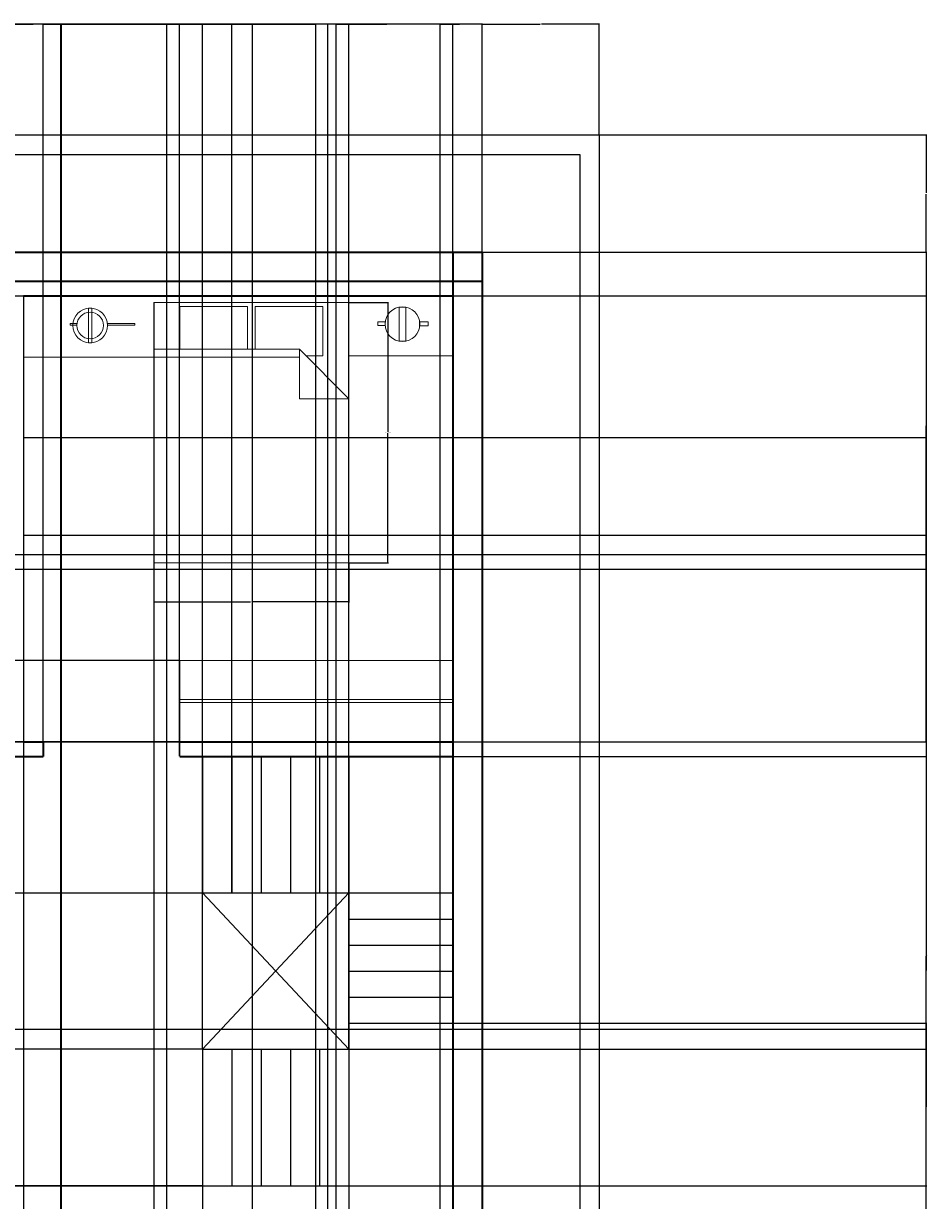
# Model space of a CAD drawing. Units: inches. Extents: x -47 to 496, y -43 to 706.
# Tile 6 of 6: x 218 to 496, y 344 to 706. Entities that reach past the tile are written whole.
import ezdxf

# ---------------------------------------------------------------- set-up
doc = ezdxf.new("R2010")
doc.units = ezdxf.units.IN
doc.linetypes.add('ACAD_ISO02W100', pattern=[15, 12, -3])
for name, color, linetype, lineweight in [('A-ANNO-DIMS', 2, 'Continuous', 18), ('A-FLOR-CASE', 3, 'Continuous', 18), ('A-FLOR-STRS-HIDN', 6, 'ACAD_ISO02W100', 18), ('C-PROP', 7, 'Continuous', 25), ('FURNITURE', 3, 'Continuous', 18), ('STAIR CASE', 6, 'Continuous', 25), ('WALL', 7, 'Continuous', 35)]:
    doc.layers.add(name, color=color, linetype=linetype, lineweight=lineweight)
doc.styles.get("Standard").update_dxf_attribs({"font": 'arial.ttf'})
doc.dimstyles.get("Standard").update_dxf_attribs({"dimtxt": 0.18, "dimasz": 0.18, "dimexe": 0.18, "dimexo": 0.0625, "dimgap": 0.09, "dimtad": 0, "dimtih": 1, "dimtoh": 1, "dimdec": 4, "dimzin": 0, "dimdsep": 46, "dimtxsty": 'Standard', "dimcen": 0.09, "dimadec": 0, "dimazin": 0, "dimtfac": 1, "dimtdec": 4, "dimtofl": 0, "dimtmove": 0, "dimatfit": 3, "dimfxl": 1, "dimtolj": 1, "dimtzin": 0, "dimarcsym": 0})

# ---------------------------------------------------------------- blocks, each defined once
blk = doc.blocks.new('Bed - Queen')
for p, q in [((0, -80.00003), (0, 0)), ((0, 0), (59.99999, 0)), ((59.99999, 0), (59.99999, -80.00003)), ((7.99999, -1.2), (28.79998, -1.2)), ((7.99999, -14.4), (7.99999, -1.2)), ((28.79998, -1.2), (28.79998, -14.4)), ((31.19999, -1.2), (51.99999, -1.2)), ((31.19999, -14.4), (31.19999, -1.2)), ((51.99999, -1.2), (51.99999, -16.4)), ((0, -14.4), (44.8, -14.4)), ((59.99999, -29.6), (44.8, -14.4)), ((44.8, -14.4), (44.8, -29.6)), ((44.8, -16.8), (0, -16.8)), ((51.99999, -16.4), (46.79936, -16.4)), ((44.8, -29.6), (59.99999, -29.6)), ((59.99999, -80.00003), (0, -80.00003))]:
    blk.add_line(p, q)
blk = doc.blocks.new('*D10')
at = {"layer": 'A-ANNO-DIMS', "color": 0, "lineweight": -2, "transparency": 16777216}
for p, q in [((318.53, 619.97), (330.64, 619.97)), ((330.46, 619.79), (330.46, 580.16)), ((330.46, 540.15), (330.46, 579.78)), ((318.53, 539.97), (330.64, 539.97))]:
    blk.add_line(p, q, dxfattribs=at)
at = {"layer": 'A-ANNO-DIMS', "color": 0, "transparency": 16777216}
for points in [[(330.43, 619.79), (330.49, 619.79), (330.46, 619.97)], [(330.43, 540.15), (330.49, 540.15), (330.46, 539.97)]]:
    blk.add_solid(points, dxfattribs=at)
at = {"layer": 'Defpoints', "color": 0, "transparency": 16777216}
for p in [(318.46, 619.97), (330.46, 619.97), (318.46, 539.97)]:
    blk.add_point(p, dxfattribs=at)
at = {"layer": 'A-ANNO-DIMS', "color": 0, "transparency": 16777216, "insert": (330.46, 579.97), "char_height": 0.18, "attachment_point": 5}
blk.add_mtext('\\A1;QUEEN BED 80', dxfattribs=at)
blk = doc.blocks.new('*D11')
at = {"layer": 'A-ANNO-DIMS', "color": 0, "lineweight": -2, "transparency": 16777216}
for p, q in [((258.46, 539.91), (258.46, 527.79)), ((318.46, 539.91), (318.46, 527.79)), ((258.64, 527.97), (288.24, 527.97)), ((318.28, 527.97), (288.68, 527.97))]:
    blk.add_line(p, q, dxfattribs=at)
at = {"layer": 'A-ANNO-DIMS', "color": 0, "transparency": 16777216}
for points in [[(258.64, 528), (258.64, 527.94), (258.46, 527.97)], [(318.28, 528), (318.28, 527.94), (318.46, 527.97)]]:
    blk.add_solid(points, dxfattribs=at)
at = {"layer": 'Defpoints', "color": 0, "transparency": 16777216}
for p in [(258.46, 539.97), (318.46, 539.97), (318.46, 527.97)]:
    blk.add_point(p, dxfattribs=at)
at = {"layer": 'A-ANNO-DIMS', "color": 0, "transparency": 16777216, "insert": (288.46, 527.97), "char_height": 0.18, "attachment_point": 5}
blk.add_mtext('\\A1;60', dxfattribs=at)
blk = doc.blocks.new('*D16')
at = {"layer": 'A-ANNO-DIMS', "color": 0, "lineweight": -2, "transparency": 16777216}
for p, q in [((359.45, 635.53), (359.45, 705.7)), ((359.63, 705.52), (377.24, 705.52)), ((395.27, 705.52), (377.67, 705.52)), ((395.45, 671.53), (395.45, 705.7))]:
    blk.add_line(p, q, dxfattribs=at)
at = {"layer": 'A-ANNO-DIMS', "color": 0, "transparency": 16777216}
for points in [[(359.63, 705.55), (359.63, 705.49), (359.45, 705.52)], [(395.27, 705.55), (395.27, 705.49), (395.45, 705.52)]]:
    blk.add_solid(points, dxfattribs=at)
at = {"layer": 'Defpoints', "color": 0, "transparency": 16777216}
for p in [(395.45, 705.52), (395.45, 671.47), (359.45, 635.47)]:
    blk.add_point(p, dxfattribs=at)
at = {"layer": 'A-ANNO-DIMS', "color": 0, "transparency": 16777216, "insert": (377.45, 705.52), "char_height": 0.18, "attachment_point": 5}
blk.add_mtext('\\A1;36', dxfattribs=at)
blk = doc.blocks.new('*D17')
at = {"layer": 'A-ANNO-DIMS', "color": 0, "lineweight": -2, "transparency": 16777216}
for p, q in [((395.52, 671.47), (496.14, 671.47)), ((495.96, 671.29), (495.96, 653.65)), ((495.96, 635.65), (495.96, 653.29)), ((359.52, 635.47), (496.14, 635.47))]:
    blk.add_line(p, q, dxfattribs=at)
at = {"layer": 'A-ANNO-DIMS', "color": 0, "transparency": 16777216}
for points in [[(495.93, 671.29), (495.99, 671.29), (495.96, 671.47)], [(495.93, 635.65), (495.99, 635.65), (495.96, 635.47)]]:
    blk.add_solid(points, dxfattribs=at)
at = {"layer": 'Defpoints', "color": 0, "transparency": 16777216}
for p in [(395.45, 671.47), (495.96, 671.47), (359.45, 635.47)]:
    blk.add_point(p, dxfattribs=at)
at = {"layer": 'A-ANNO-DIMS', "color": 0, "transparency": 16777216, "insert": (495.96, 653.47), "char_height": 0.18, "attachment_point": 5}
blk.add_mtext('\\A1;36', dxfattribs=at)
blk = doc.blocks.new('*D18')
at = {"layer": 'A-ANNO-DIMS', "color": 0, "lineweight": -2, "transparency": 16777216}
for p, q in [((359.52, 635.47), (496.14, 635.47)), ((495.96, 635.29), (495.96, 419.4)), ((495.96, 203.15), (495.96, 419.04)), ((359.52, 202.97), (496.14, 202.97))]:
    blk.add_line(p, q, dxfattribs=at)
at = {"layer": 'A-ANNO-DIMS', "color": 0, "transparency": 16777216}
for points in [[(495.93, 635.29), (495.99, 635.29), (495.96, 635.47)], [(495.93, 203.15), (495.99, 203.15), (495.96, 202.97)]]:
    blk.add_solid(points, dxfattribs=at)
at = {"layer": 'Defpoints', "color": 0, "transparency": 16777216}
for p in [(359.45, 635.47), (495.96, 635.47), (359.45, 202.97)]:
    blk.add_point(p, dxfattribs=at)
at = {"layer": 'A-ANNO-DIMS', "color": 0, "transparency": 16777216, "insert": (495.96, 419.22), "char_height": 0.18, "attachment_point": 5}
blk.add_mtext('\\A1;432.5', dxfattribs=at)
blk = doc.blocks.new('*D22')
at = {"layer": 'A-ANNO-DIMS', "color": 0, "lineweight": -2, "transparency": 16777216}
for p, q in [((229.88, 163.9), (229.88, 705.7)), ((230.06, 705.52), (245.73, 705.52)), ((262.33, 705.52), (246.66, 705.52)), ((262.51, 163.9), (262.51, 705.7))]:
    blk.add_line(p, q, dxfattribs=at)
at = {"layer": 'A-ANNO-DIMS', "color": 0, "transparency": 16777216}
for points in [[(230.06, 705.55), (230.06, 705.49), (229.88, 705.52)], [(262.33, 705.55), (262.33, 705.49), (262.51, 705.52)]]:
    blk.add_solid(points, dxfattribs=at)
at = {"layer": 'Defpoints', "color": 0, "transparency": 16777216}
for p in [(262.51, 705.52), (229.88, 163.83), (262.51, 163.83)]:
    blk.add_point(p, dxfattribs=at)
at = {"layer": 'A-ANNO-DIMS', "color": 0, "transparency": 16777216, "insert": (246.2, 705.52), "char_height": 0.18, "attachment_point": 5}
blk.add_mtext('\\A1;32.636', dxfattribs=at)
blk = doc.blocks.new('*D24')
at = {"layer": 'A-ANNO-DIMS', "color": 0, "lineweight": -2, "transparency": 16777216}
for p, q in [((314.53, 186.25), (314.53, 705.7)), ((314.71, 705.52), (330.12, 705.52)), ((346.32, 705.52), (330.91, 705.52)), ((346.5, 186.25), (346.5, 705.7))]:
    blk.add_line(p, q, dxfattribs=at)
at = {"layer": 'A-ANNO-DIMS', "color": 0, "transparency": 16777216}
for points in [[(314.71, 705.55), (314.71, 705.49), (314.53, 705.52)], [(346.32, 705.55), (346.32, 705.49), (346.5, 705.52)]]:
    blk.add_solid(points, dxfattribs=at)
at = {"layer": 'Defpoints', "color": 0, "transparency": 16777216}
for p in [(346.5, 705.52), (314.53, 186.18), (346.5, 186.18)]:
    blk.add_point(p, dxfattribs=at)
at = {"layer": 'A-ANNO-DIMS', "color": 0, "transparency": 16777216, "insert": (330.52, 705.52), "char_height": 0.18, "attachment_point": 5}
blk.add_mtext('\\A1;31.97', dxfattribs=at)
blk = doc.blocks.new('*D26')
at = {"layer": 'A-ANNO-DIMS', "color": 0, "lineweight": -2, "transparency": 16777216}
for p, q in [((213.95, 131.03), (213.95, 705.7)), ((214.13, 705.52), (221.46, 705.52)), ((229.7, 705.52), (222.37, 705.52)), ((229.88, 163.9), (229.88, 705.7))]:
    blk.add_line(p, q, dxfattribs=at)
at = {"layer": 'A-ANNO-DIMS', "color": 0, "transparency": 16777216}
for points in [[(214.13, 705.55), (214.13, 705.49), (213.95, 705.52)], [(229.7, 705.55), (229.7, 705.49), (229.88, 705.52)]]:
    blk.add_solid(points, dxfattribs=at)
at = {"layer": 'Defpoints', "color": 0, "transparency": 16777216}
for p in [(229.88, 705.52), (229.88, 163.83), (213.95, 130.97)]:
    blk.add_point(p, dxfattribs=at)
at = {"layer": 'A-ANNO-DIMS', "color": 0, "transparency": 16777216, "insert": (221.92, 705.52), "char_height": 0.18, "attachment_point": 5}
blk.add_mtext('\\A1;15.924', dxfattribs=at)
blk = doc.blocks.new('*D28')
at = {"layer": 'A-ANNO-DIMS', "color": 0, "lineweight": -2, "transparency": 16777216}
for p, q in [((346.5, 165.93), (346.5, 705.7)), ((346.68, 705.52), (352.52, 705.52)), ((359.27, 705.52), (353.43, 705.52)), ((359.45, 131.03), (359.45, 705.7))]:
    blk.add_line(p, q, dxfattribs=at)
at = {"layer": 'A-ANNO-DIMS', "color": 0, "transparency": 16777216}
for points in [[(346.68, 705.55), (346.68, 705.49), (346.5, 705.52)], [(359.27, 705.55), (359.27, 705.49), (359.45, 705.52)]]:
    blk.add_solid(points, dxfattribs=at)
at = {"layer": 'Defpoints', "color": 0, "transparency": 16777216}
for p in [(359.45, 705.52), (346.5, 165.87), (359.45, 130.97)]:
    blk.add_point(p, dxfattribs=at)
at = {"layer": 'A-ANNO-DIMS', "color": 0, "transparency": 16777216, "insert": (352.98, 705.52), "char_height": 0.18, "attachment_point": 5}
blk.add_mtext('\\A1;12.954', dxfattribs=at)
blk = doc.blocks.new('*D32')
at = {"layer": 'A-ANNO-DIMS', "color": 0, "lineweight": -2, "transparency": 16777216}
for p, q in [((61.45, 635.53), (61.45, 705.7)), ((61.63, 705.52), (210.16, 705.52)), ((359.27, 705.52), (210.75, 705.52)), ((359.45, 635.53), (359.45, 705.7))]:
    blk.add_line(p, q, dxfattribs=at)
at = {"layer": 'A-ANNO-DIMS', "color": 0, "transparency": 16777216}
for points in [[(61.63, 705.55), (61.63, 705.49), (61.45, 705.52)], [(359.27, 705.55), (359.27, 705.49), (359.45, 705.52)]]:
    blk.add_solid(points, dxfattribs=at)
at = {"layer": 'Defpoints', "color": 0, "transparency": 16777216}
for p in [(359.45, 705.52), (61.45, 635.47), (359.45, 635.47)]:
    blk.add_point(p, dxfattribs=at)
at = {"layer": 'A-ANNO-DIMS', "color": 0, "transparency": 16777216, "insert": (210.45, 705.52), "char_height": 0.18, "attachment_point": 5}
blk.add_mtext('\\A1;298', dxfattribs=at)
blk = doc.blocks.new('*D35')
at = {"layer": 'A-ANNO-DIMS', "color": 0, "lineweight": -2, "transparency": 16777216}
for p, q in [((218.45, 484.91), (218.45, -42.84)), ((350.45, 480.41), (350.45, -42.84)), ((218.63, -42.66), (284.18, -42.66)), ((350.27, -42.66), (284.73, -42.66))]:
    blk.add_line(p, q, dxfattribs=at)
at = {"layer": 'A-ANNO-DIMS', "color": 0, "transparency": 16777216}
for points in [[(218.63, -42.63), (218.63, -42.69), (218.45, -42.66)], [(350.27, -42.63), (350.27, -42.69), (350.45, -42.66)]]:
    blk.add_solid(points, dxfattribs=at)
at = {"layer": 'Defpoints', "color": 0, "transparency": 16777216}
for p in [(218.45, 484.97), (350.45, 480.47), (350.45, -42.66)]:
    blk.add_point(p, dxfattribs=at)
at = {"layer": 'A-ANNO-DIMS', "color": 0, "transparency": 16777216, "insert": (284.45, -42.66), "char_height": 0.18, "attachment_point": 5}
blk.add_mtext('\\A1;132', dxfattribs=at)
blk = doc.blocks.new('*D36')
at = {"layer": 'A-ANNO-DIMS', "color": 0, "lineweight": -2, "transparency": 16777216}
for p, q in [((70.52, 621.97), (496.14, 621.97)), ((495.96, 621.79), (495.96, 553.65)), ((495.96, 485.15), (495.96, 553.29)), ((70.52, 484.97), (496.14, 484.97))]:
    blk.add_line(p, q, dxfattribs=at)
at = {"layer": 'A-ANNO-DIMS', "color": 0, "transparency": 16777216}
for points in [[(495.93, 621.79), (495.99, 621.79), (495.96, 621.97)], [(495.93, 485.15), (495.99, 485.15), (495.96, 484.97)]]:
    blk.add_solid(points, dxfattribs=at)
at = {"layer": 'Defpoints', "color": 0, "transparency": 16777216}
for p in [(70.45, 621.97), (495.96, 621.97), (70.45, 484.97)]:
    blk.add_point(p, dxfattribs=at)
at = {"layer": 'A-ANNO-DIMS', "color": 0, "transparency": 16777216, "insert": (495.96, 553.47), "char_height": 0.18, "attachment_point": 5}
blk.add_mtext('\\A1;137', dxfattribs=at)
blk = doc.blocks.new('*D37')
at = {"layer": 'A-ANNO-DIMS', "color": 0, "lineweight": -2, "transparency": 16777216}
for p, q in [((166.02, 621.97), (496.14, 621.97)), ((495.96, 621.79), (495.96, 582.4)), ((495.96, 542.65), (495.96, 582.04)), ((166.02, 542.47), (496.14, 542.47))]:
    blk.add_line(p, q, dxfattribs=at)
at = {"layer": 'A-ANNO-DIMS', "color": 0, "transparency": 16777216}
for points in [[(495.93, 621.79), (495.99, 621.79), (495.96, 621.97)], [(495.93, 542.65), (495.99, 542.65), (495.96, 542.47)]]:
    blk.add_solid(points, dxfattribs=at)
at = {"layer": 'Defpoints', "color": 0, "transparency": 16777216}
for p in [(165.95, 621.97), (495.96, 621.97), (165.95, 542.47)]:
    blk.add_point(p, dxfattribs=at)
at = {"layer": 'A-ANNO-DIMS', "color": 0, "transparency": 16777216, "insert": (495.96, 582.22), "char_height": 0.18, "attachment_point": 5}
blk.add_mtext('\\A1;79.5', dxfattribs=at)
blk = doc.blocks.new('*D38')
at = {"layer": 'A-ANNO-DIMS', "color": 0, "lineweight": -2, "transparency": 16777216}
for p, q in [((166.02, 537.97), (496.14, 537.97)), ((495.96, 537.79), (495.96, 511.65)), ((495.96, 485.15), (495.96, 511.29)), ((166.02, 484.97), (496.14, 484.97))]:
    blk.add_line(p, q, dxfattribs=at)
at = {"layer": 'A-ANNO-DIMS', "color": 0, "transparency": 16777216}
for points in [[(495.93, 537.79), (495.99, 537.79), (495.96, 537.97)], [(495.93, 485.15), (495.99, 485.15), (495.96, 484.97)]]:
    blk.add_solid(points, dxfattribs=at)
at = {"layer": 'Defpoints', "color": 0, "transparency": 16777216}
for p in [(165.95, 537.97), (495.96, 537.97), (165.95, 484.97)]:
    blk.add_point(p, dxfattribs=at)
at = {"layer": 'A-ANNO-DIMS', "color": 0, "transparency": 16777216, "insert": (495.96, 511.47), "char_height": 0.18, "attachment_point": 5}
blk.add_mtext('\\A1;53', dxfattribs=at)
blk = doc.blocks.new('*D39')
at = {"layer": 'A-ANNO-DIMS', "color": 0, "lineweight": -2, "transparency": 16777216}
for p, q in [((218.52, 578.47), (496.14, 578.47)), ((495.96, 578.29), (495.96, 563.65)), ((495.96, 548.65), (495.96, 563.29)), ((218.52, 548.47), (496.14, 548.47))]:
    blk.add_line(p, q, dxfattribs=at)
at = {"layer": 'A-ANNO-DIMS', "color": 0, "transparency": 16777216}
for points in [[(495.93, 578.29), (495.99, 578.29), (495.96, 578.47)], [(495.93, 548.65), (495.99, 548.65), (495.96, 548.47)]]:
    blk.add_solid(points, dxfattribs=at)
at = {"layer": 'Defpoints', "color": 0, "transparency": 16777216}
for p in [(218.45, 578.47), (495.96, 578.47), (218.45, 548.47)]:
    blk.add_point(p, dxfattribs=at)
at = {"layer": 'A-ANNO-DIMS', "color": 0, "transparency": 16777216, "insert": (495.96, 563.47), "char_height": 0.18, "attachment_point": 5}
blk.add_mtext('\\A1;30', dxfattribs=at)
blk = doc.blocks.new('*D48')
at = {"layer": 'A-ANNO-DIMS', "color": 0, "lineweight": -2, "transparency": 16777216}
for p, q in [((224.45, 480.53), (224.45, 705.7)), ((224.63, 705.52), (245.23, 705.52)), ((266.27, 705.52), (245.68, 705.52)), ((266.45, 480.53), (266.45, 705.7))]:
    blk.add_line(p, q, dxfattribs=at)
at = {"layer": 'A-ANNO-DIMS', "color": 0, "transparency": 16777216}
for points in [[(224.63, 705.55), (224.63, 705.49), (224.45, 705.52)], [(266.27, 705.55), (266.27, 705.49), (266.45, 705.52)]]:
    blk.add_solid(points, dxfattribs=at)
at = {"layer": 'Defpoints', "color": 0, "transparency": 16777216}
for p in [(266.45, 705.52), (224.45, 480.47), (266.45, 480.47)]:
    blk.add_point(p, dxfattribs=at)
at = {"layer": 'A-ANNO-DIMS', "color": 0, "transparency": 16777216, "insert": (245.45, 705.52), "char_height": 0.18, "attachment_point": 5}
blk.add_mtext('\\A1;42', dxfattribs=at)
blk = doc.blocks.new('*D51')
at = {"layer": 'A-ANNO-DIMS', "color": 0, "lineweight": -2, "transparency": 16777216}
for p, q in [((218.45, 621.91), (218.45, -42.84)), ((258.46, 619.91), (258.46, -42.84)), ((218.63, -42.66), (238.08, -42.66)), ((258.28, -42.66), (238.84, -42.66))]:
    blk.add_line(p, q, dxfattribs=at)
at = {"layer": 'A-ANNO-DIMS', "color": 0, "transparency": 16777216}
for points in [[(218.63, -42.63), (218.63, -42.69), (218.45, -42.66)], [(258.28, -42.63), (258.28, -42.69), (258.46, -42.66)]]:
    blk.add_solid(points, dxfattribs=at)
at = {"layer": 'Defpoints', "color": 0, "transparency": 16777216}
for p in [(218.45, 621.97), (258.46, 619.97), (258.46, -42.66)]:
    blk.add_point(p, dxfattribs=at)
at = {"layer": 'A-ANNO-DIMS', "color": 0, "transparency": 16777216, "insert": (238.46, -42.66), "char_height": 0.18, "attachment_point": 5}
blk.add_mtext('\\A1;40.01', dxfattribs=at)
blk = doc.blocks.new('*D52')
at = {"layer": 'A-ANNO-DIMS', "color": 0, "lineweight": -2, "transparency": 16777216}
for p, q in [((266.45, 510.03), (266.45, 705.7)), ((266.63, 705.52), (308.24, 705.52)), ((350.27, 705.52), (308.67, 705.52)), ((350.45, 510.03), (350.45, 705.7))]:
    blk.add_line(p, q, dxfattribs=at)
at = {"layer": 'A-ANNO-DIMS', "color": 0, "transparency": 16777216}
for points in [[(266.63, 705.55), (266.63, 705.49), (266.45, 705.52)], [(350.27, 705.55), (350.27, 705.49), (350.45, 705.52)]]:
    blk.add_solid(points, dxfattribs=at)
at = {"layer": 'Defpoints', "color": 0, "transparency": 16777216}
for p in [(350.45, 705.52), (266.45, 509.97), (350.45, 509.97)]:
    blk.add_point(p, dxfattribs=at)
at = {"layer": 'A-ANNO-DIMS', "color": 0, "transparency": 16777216, "insert": (308.45, 705.52), "char_height": 0.18, "attachment_point": 5}
blk.add_mtext('\\A1;84', dxfattribs=at)
blk = doc.blocks.new('*D53')
at = {"layer": 'A-ANNO-DIMS', "color": 0, "lineweight": -2, "transparency": 16777216}
for p, q in [((266.39, 509.97), (-47.29, 509.97)), ((-47.11, 509.79), (-47.11, 497.65)), ((-47.11, 485.15), (-47.11, 497.29)), ((266.39, 484.97), (-47.29, 484.97))]:
    blk.add_line(p, q, dxfattribs=at)
at = {"layer": 'A-ANNO-DIMS', "color": 0, "transparency": 16777216}
for points in [[(-47.14, 509.79), (-47.08, 509.79), (-47.11, 509.97)], [(-47.14, 485.15), (-47.08, 485.15), (-47.11, 484.97)]]:
    blk.add_solid(points, dxfattribs=at)
at = {"layer": 'Defpoints', "color": 0, "transparency": 16777216}
for p in [(-47.11, 509.97), (266.45, 509.97), (266.45, 484.97)]:
    blk.add_point(p, dxfattribs=at)
at = {"layer": 'A-ANNO-DIMS', "color": 0, "transparency": 16777216, "insert": (-47.11, 497.47), "char_height": 0.18, "attachment_point": 5}
blk.add_mtext('\\A1;25', dxfattribs=at)
blk = doc.blocks.new('*D54')
at = {"layer": 'A-ANNO-DIMS', "color": 0, "lineweight": -2, "transparency": 16777216}
for p, q in [((273.48, 348.41), (273.48, -42.84)), ((350.45, 348.41), (350.45, -42.84)), ((273.66, -42.66), (311.57, -42.66)), ((350.27, -42.66), (312.36, -42.66))]:
    blk.add_line(p, q, dxfattribs=at)
at = {"layer": 'A-ANNO-DIMS', "color": 0, "transparency": 16777216}
for points in [[(273.66, -42.63), (273.66, -42.69), (273.48, -42.66)], [(350.27, -42.63), (350.27, -42.69), (350.45, -42.66)]]:
    blk.add_solid(points, dxfattribs=at)
at = {"layer": 'Defpoints', "color": 0, "transparency": 16777216}
for p in [(273.48, 348.47), (350.45, 348.47), (350.45, -42.66)]:
    blk.add_point(p, dxfattribs=at)
at = {"layer": 'A-ANNO-DIMS', "color": 0, "transparency": 16777216, "insert": (311.97, -42.66), "char_height": 0.18, "attachment_point": 5}
blk.add_mtext('\\A1;76.97', dxfattribs=at)
blk = doc.blocks.new('*D55')
at = {"layer": 'A-ANNO-DIMS', "color": 0, "lineweight": -2, "transparency": 16777216}
for p, q in [((350.52, 480.47), (496.14, 480.47)), ((495.96, 480.29), (495.96, 414.65)), ((495.96, 348.65), (495.96, 414.29)), ((350.52, 348.47), (496.14, 348.47))]:
    blk.add_line(p, q, dxfattribs=at)
at = {"layer": 'A-ANNO-DIMS', "color": 0, "transparency": 16777216}
for points in [[(495.93, 480.29), (495.99, 480.29), (495.96, 480.47)], [(495.93, 348.65), (495.99, 348.65), (495.96, 348.47)]]:
    blk.add_solid(points, dxfattribs=at)
at = {"layer": 'Defpoints', "color": 0, "transparency": 16777216}
for p in [(350.45, 480.47), (495.96, 480.47), (350.45, 348.47)]:
    blk.add_point(p, dxfattribs=at)
at = {"layer": 'A-ANNO-DIMS', "color": 0, "transparency": 16777216, "insert": (495.96, 414.47), "char_height": 0.18, "attachment_point": 5}
blk.add_mtext('\\A1;132', dxfattribs=at)
blk = doc.blocks.new('*D56')
at = {"layer": 'A-ANNO-DIMS', "color": 0, "lineweight": -2, "transparency": 16777216}
for p, q in [((273.48, 390.53), (273.48, 705.7)), ((273.66, 705.52), (295.76, 705.52)), ((318.3, 705.52), (296.2, 705.52)), ((318.48, 390.53), (318.48, 705.7))]:
    blk.add_line(p, q, dxfattribs=at)
at = {"layer": 'A-ANNO-DIMS', "color": 0, "transparency": 16777216}
for points in [[(273.66, 705.55), (273.66, 705.49), (273.48, 705.52)], [(318.3, 705.55), (318.3, 705.49), (318.48, 705.52)]]:
    blk.add_solid(points, dxfattribs=at)
at = {"layer": 'Defpoints', "color": 0, "transparency": 16777216}
for p in [(318.48, 705.52), (273.48, 390.47), (318.48, 390.47)]:
    blk.add_point(p, dxfattribs=at)
at = {"layer": 'A-ANNO-DIMS', "color": 0, "transparency": 16777216, "insert": (295.98, 705.52), "char_height": 0.18, "attachment_point": 5}
blk.add_mtext('\\A1;45', dxfattribs=at)
blk = doc.blocks.new('*D57')
at = {"layer": 'A-ANNO-DIMS', "color": 0, "lineweight": -2, "transparency": 16777216}
for p, q in [((273.42, 438.47), (-47.29, 438.47)), ((-47.11, 438.29), (-47.11, 414.65)), ((-47.11, 390.65), (-47.11, 414.29)), ((273.42, 390.47), (-47.29, 390.47))]:
    blk.add_line(p, q, dxfattribs=at)
at = {"layer": 'A-ANNO-DIMS', "color": 0, "transparency": 16777216}
for points in [[(-47.14, 438.29), (-47.08, 438.29), (-47.11, 438.47)], [(-47.14, 390.65), (-47.08, 390.65), (-47.11, 390.47)]]:
    blk.add_solid(points, dxfattribs=at)
at = {"layer": 'Defpoints', "color": 0, "transparency": 16777216}
for p in [(-47.11, 438.47), (273.48, 438.47), (273.48, 390.47)]:
    blk.add_point(p, dxfattribs=at)
at = {"layer": 'A-ANNO-DIMS', "color": 0, "transparency": 16777216, "insert": (-47.11, 414.47), "char_height": 0.18, "attachment_point": 5}
blk.add_mtext('\\A1;48', dxfattribs=at)
blk = doc.blocks.new('*D58')
at = {"layer": 'A-ANNO-DIMS', "color": 0, "lineweight": -2, "transparency": 16777216}
for p, q in [((273.42, 390.47), (-47.29, 390.47)), ((-47.11, 390.29), (-47.11, 369.65)), ((-47.11, 348.65), (-47.11, 369.29)), ((273.42, 348.47), (-47.29, 348.47))]:
    blk.add_line(p, q, dxfattribs=at)
at = {"layer": 'A-ANNO-DIMS', "color": 0, "transparency": 16777216}
for points in [[(-47.14, 390.29), (-47.08, 390.29), (-47.11, 390.47)], [(-47.14, 348.65), (-47.08, 348.65), (-47.11, 348.47)]]:
    blk.add_solid(points, dxfattribs=at)
at = {"layer": 'Defpoints', "color": 0, "transparency": 16777216}
for p in [(-47.11, 390.47), (273.48, 390.47), (273.48, 348.47)]:
    blk.add_point(p, dxfattribs=at)
at = {"layer": 'A-ANNO-DIMS', "color": 0, "transparency": 16777216, "insert": (-47.11, 369.47), "char_height": 0.18, "attachment_point": 5}
blk.add_mtext('\\A1;42', dxfattribs=at)
blk = doc.blocks.new('*D59')
at = {"layer": 'A-ANNO-DIMS', "color": 0, "lineweight": -2, "transparency": 16777216}
for p, q in [((318.48, 390.41), (318.48, -42.84)), ((350.45, 390.41), (350.45, -42.84)), ((318.66, -42.66), (334, -42.66)), ((350.27, -42.66), (334.93, -42.66))]:
    blk.add_line(p, q, dxfattribs=at)
at = {"layer": 'A-ANNO-DIMS', "color": 0, "transparency": 16777216}
for points in [[(318.66, -42.63), (318.66, -42.69), (318.48, -42.66)], [(350.27, -42.63), (350.27, -42.69), (350.45, -42.66)]]:
    blk.add_solid(points, dxfattribs=at)
at = {"layer": 'Defpoints', "color": 0, "transparency": 16777216}
for p in [(318.48, 390.47), (350.45, 390.47), (350.45, -42.66)]:
    blk.add_point(p, dxfattribs=at)
at = {"layer": 'A-ANNO-DIMS', "color": 0, "transparency": 16777216, "insert": (334.47, -42.66), "char_height": 0.18, "attachment_point": 5}
blk.add_mtext('\\A1;31.975', dxfattribs=at)
blk = doc.blocks.new('*D60')
at = {"layer": 'A-ANNO-DIMS', "color": 0, "lineweight": -2, "transparency": 16777216}
for p, q in [((273.48, 438.53), (273.48, 705.7)), ((273.66, 705.52), (277.83, 705.52)), ((282.3, 705.52), (278.13, 705.52)), ((282.48, 438.53), (282.48, 705.7))]:
    blk.add_line(p, q, dxfattribs=at)
at = {"layer": 'A-ANNO-DIMS', "color": 0, "transparency": 16777216}
for points in [[(273.66, 705.55), (273.66, 705.49), (273.48, 705.52)], [(282.3, 705.55), (282.3, 705.49), (282.48, 705.52)]]:
    blk.add_solid(points, dxfattribs=at)
at = {"layer": 'Defpoints', "color": 0, "transparency": 16777216}
for p in [(282.48, 705.52), (273.48, 438.47), (282.48, 438.47)]:
    blk.add_point(p, dxfattribs=at)
at = {"layer": 'A-ANNO-DIMS', "color": 0, "transparency": 16777216, "insert": (277.98, 705.52), "char_height": 0.18, "attachment_point": 5}
blk.add_mtext('\\A1;9', dxfattribs=at)
blk = doc.blocks.new('*D61')
at = {"layer": 'A-ANNO-DIMS', "color": 0, "lineweight": -2, "transparency": 16777216}
for p, q in [((318.54, 398.47), (496.14, 398.47)), ((495.96, 398.29), (495.96, 394.65)), ((495.96, 390.65), (495.96, 394.29)), ((318.54, 390.47), (496.14, 390.47))]:
    blk.add_line(p, q, dxfattribs=at)
at = {"layer": 'A-ANNO-DIMS', "color": 0, "transparency": 16777216}
for points in [[(495.93, 398.29), (495.99, 398.29), (495.96, 398.47)], [(495.93, 390.65), (495.99, 390.65), (495.96, 390.47)]]:
    blk.add_solid(points, dxfattribs=at)
at = {"layer": 'Defpoints', "color": 0, "transparency": 16777216}
for p in [(318.48, 398.47), (495.96, 398.47), (318.48, 390.47)]:
    blk.add_point(p, dxfattribs=at)
at = {"layer": 'A-ANNO-DIMS', "color": 0, "transparency": 16777216, "insert": (495.96, 394.47), "char_height": 0.18, "attachment_point": 5}
blk.add_mtext('\\A1;8', dxfattribs=at)
blk = doc.blocks.new('*D65')
at = {"layer": 'A-ANNO-DIMS', "color": 0, "lineweight": -2, "transparency": 16777216}
for p, q in [((218.45, 348.41), (218.45, -42.84)), ((273.48, 348.41), (273.48, -42.84)), ((218.63, -42.66), (245.57, -42.66)), ((273.3, -42.66), (246.36, -42.66))]:
    blk.add_line(p, q, dxfattribs=at)
at = {"layer": 'A-ANNO-DIMS', "color": 0, "transparency": 16777216}
for points in [[(218.63, -42.63), (218.63, -42.69), (218.45, -42.66)], [(273.3, -42.63), (273.3, -42.69), (273.48, -42.66)]]:
    blk.add_solid(points, dxfattribs=at)
at = {"layer": 'Defpoints', "color": 0, "transparency": 16777216}
for p in [(218.45, 348.47), (273.48, 348.47), (273.48, -42.66)]:
    blk.add_point(p, dxfattribs=at)
at = {"layer": 'A-ANNO-DIMS', "color": 0, "transparency": 16777216, "insert": (245.97, -42.66), "char_height": 0.18, "attachment_point": 5}
blk.add_mtext('\\A1;55.03', dxfattribs=at)
blk = doc.blocks.new('*D69')
at = {"layer": 'A-ANNO-DIMS', "color": 0, "lineweight": -2, "transparency": 16777216}
for p, q in [((180.11, 396.63), (496.14, 396.63)), ((495.96, 396.45), (495.96, 372.73)), ((495.96, 348.65), (495.96, 372.37)), ((158.09, 348.47), (496.14, 348.47))]:
    blk.add_line(p, q, dxfattribs=at)
at = {"layer": 'A-ANNO-DIMS', "color": 0, "transparency": 16777216}
for points in [[(495.93, 396.45), (495.99, 396.45), (495.96, 396.63)], [(495.93, 348.65), (495.99, 348.65), (495.96, 348.47)]]:
    blk.add_solid(points, dxfattribs=at)
at = {"layer": 'Defpoints', "color": 0, "transparency": 16777216}
for p in [(180.05, 396.63), (158.02, 348.47), (495.96, 348.47)]:
    blk.add_point(p, dxfattribs=at)
at = {"layer": 'A-ANNO-DIMS', "color": 0, "transparency": 16777216, "insert": (495.96, 372.55), "char_height": 0.18, "attachment_point": 5}
blk.add_mtext('\\A1;48.155', dxfattribs=at)
blk = doc.blocks.new('*D78')
at = {"layer": 'A-ANNO-DIMS', "color": 0, "lineweight": -2, "transparency": 16777216}
for p, q in [((230.13, 246.14), (230.13, 705.7)), ((230.31, 705.52), (270.64, 705.52)), ((311.77, 705.52), (271.43, 705.52)), ((311.95, 246.14), (311.95, 705.7))]:
    blk.add_line(p, q, dxfattribs=at)
at = {"layer": 'A-ANNO-DIMS', "color": 0, "transparency": 16777216}
for points in [[(230.31, 705.55), (230.31, 705.49), (230.13, 705.52)], [(311.77, 705.55), (311.77, 705.49), (311.95, 705.52)]]:
    blk.add_solid(points, dxfattribs=at)
at = {"layer": 'Defpoints', "color": 0, "transparency": 16777216}
for p in [(311.95, 705.52), (230.13, 246.07), (311.95, 246.07)]:
    blk.add_point(p, dxfattribs=at)
at = {"layer": 'A-ANNO-DIMS', "color": 0, "transparency": 16777216, "insert": (271.04, 705.52), "char_height": 0.18, "attachment_point": 5}
blk.add_mtext('\\A1;81.82', dxfattribs=at)
blk = doc.blocks.new('*D86')
at = {"layer": 'A-ANNO-DIMS', "color": 0, "lineweight": -2, "transparency": 16777216}
for p, q in [((288.82, 318.79), (288.82, 705.7)), ((289, 705.52), (298.16, 705.52)), ((308.09, 705.52), (298.93, 705.52)), ((308.27, 318.79), (308.27, 705.7))]:
    blk.add_line(p, q, dxfattribs=at)
at = {"layer": 'A-ANNO-DIMS', "color": 0, "transparency": 16777216}
for points in [[(289, 705.55), (289, 705.49), (288.82, 705.52)], [(308.09, 705.55), (308.09, 705.49), (308.27, 705.52)]]:
    blk.add_solid(points, dxfattribs=at)
at = {"layer": 'Defpoints', "color": 0, "transparency": 16777216}
for p in [(308.27, 705.52), (288.82, 318.72), (308.27, 318.72)]:
    blk.add_point(p, dxfattribs=at)
at = {"layer": 'A-ANNO-DIMS', "color": 0, "transparency": 16777216, "insert": (298.54, 705.52), "char_height": 0.18, "attachment_point": 5}
blk.add_mtext('\\A1;19.45', dxfattribs=at)

msp = doc.modelspace()

# ---------------------------------------------------------------- linework, layer by layer
at = {"layer": 'A-FLOR-CASE'}
for p, q in [((266.4545, 509.9711), (266.4545, 480.4711)), ((266.4545, 509.9711), (350.4545, 509.9711)), ((266.4545, 497.9711), (350.4545, 497.9711)), ((266.4545, 496.9711), (350.4545, 496.9711))]:
    msp.add_line(p, q, dxfattribs=at)
at = {"layer": 'A-FLOR-STRS-HIDN'}
msp.add_line((273.4798, 438.4711), (273.4798, 390.4711), dxfattribs=at)
at = {"layer": 'C-PROP'}
for p, q in [((25.4545, 671.4711), (395.4545, 671.4711)), ((395.4545, 671.4711), (395.4545, 52.9711)), ((31.4545, 665.4711), (389.4545, 665.4711)), ((389.4545, 665.4711), (389.4545, 58.9711))]:
    msp.add_line(p, q, dxfattribs=at)
at = {"layer": 'FURNITURE'}
for p, q in [((258.4632, 603.1711), (218.4545, 603.1711)), ((318.4632, 603.5711), (350.4545, 603.5711))]:
    msp.add_line(p, q, dxfattribs=at)
for points in [[(238.4127, 618.23), (239.4384, 618.23), (239.4384, 607.5739), (238.4127, 607.5739)], [(333.908, 618.557), (335.9431, 618.557), (335.9431, 608.0469), (333.908, 608.0469)], [(232.7516, 613.4643), (234.8541, 613.4643), (234.8541, 613.0358), (232.7516, 613.0358)], [(244.2486, 613.4643), (252.6303, 613.4643), (252.6303, 612.9772), (244.2486, 612.9772)], [(329.6277, 614.0661), (327.3637, 614.0661), (327.3637, 612.883), (329.6277, 612.883)], [(340.2234, 614.0661), (342.7999, 614.0661), (342.7999, 612.8122), (340.2234, 612.8122)]]:
    msp.add_lwpolyline(points, close=True, dxfattribs=at)
for centre, radius in [((334.9256, 613.3019), 5.3527), ((238.9256, 612.9019), 5.3527), ((238.9256, 612.9019), 5.3527), ((238.9256, 612.9019), 5.3527), ((238.9256, 612.9019), 4.0736)]:
    msp.add_circle(centre, radius, dxfattribs=at)
at = {"layer": 'STAIR CASE'}
for p, q in [((273.4798, 480.4711), (273.4798, 438.4711)), ((282.4798, 480.4711), (282.4798, 438.4711)), ((291.4798, 480.4711), (291.4798, 438.4711)), ((300.4798, 480.4711), (300.4798, 438.4711)), ((309.4798, 480.4711), (309.4798, 438.4711)), ((318.4798, 480.4711), (318.4798, 438.4711)), ((273.4798, 438.4711), (350.4545, 438.4711)), ((273.4798, 390.4711), (318.4798, 438.4711)), ((318.4798, 390.4711), (273.4798, 438.4711)), ((318.4798, 438.4711), (318.4798, 390.4711)), ((318.4798, 430.4711), (350.4545, 430.4711)), ((318.4798, 422.4711), (350.4545, 422.4711)), ((318.4798, 414.4711), (350.4545, 414.4711)), ((318.4798, 406.4711), (350.4545, 406.4711)), ((318.4798, 398.4711), (350.4545, 398.4711)), ((273.4798, 390.4711), (350.4545, 390.4711)), ((273.4798, 390.4711), (273.4798, 348.4711)), ((282.4798, 390.4711), (282.4798, 348.4711)), ((291.4798, 390.4711), (291.4798, 348.4711)), ((300.4798, 390.4711), (300.4798, 348.4711)), ((309.4798, 390.4711), (309.4798, 348.4711)), ((318.4798, 390.4711), (318.4798, 348.4711)), ((273.4798, 348.4711), (350.4545, 348.4711))]:
    msp.add_line(p, q, dxfattribs=at)
for p in [(318.4798, 430.4711), (318.4798, 422.4711), (318.4798, 414.4711), (318.4798, 406.4711), (318.4798, 398.4711)]:
    msp.add_point(p, dxfattribs=at)
at = {"layer": 'WALL'}
for p, q in [((61.4545, 635.4711), (359.4545, 635.4711)), ((350.4545, 635.4711), (350.4545, 202.9711)), ((359.4545, 635.4711), (359.4545, 130.9711)), ((138.255, 626.4711), (359.4545, 626.4711)), ((218.4545, 621.9711), (350.4545, 621.9711)), ((218.4545, 484.9711), (224.4545, 484.9711)), ((224.4545, 484.9711), (224.4545, 480.4711)), ((266.4545, 484.9711), (350.4545, 484.9711)), ((201.9545, 480.4711), (224.4545, 480.4711)), ((266.4545, 480.4711), (350.4545, 480.4711))]:
    msp.add_line(p, q, dxfattribs=at)

# ---------------------------------------------------------------- block references
at = {"layer": 'FURNITURE'}
msp.add_blockref('Bed - Queen', (258.4632, 619.9711), dxfattribs=at)

# ---------------------------------------------------------------- dimensions: what is measured, and where the dimension line sits
at = {"layer": 'A-ANNO-DIMS'}
for base, p1, p2, override, picture, middle in [((359.4545, 705.5211), (61.4545, 635.4711), (359.4545, 635.4711), {"dimdec": 0, "dimlfac": 1, "dimrnd": 0, "dimzin": 0, "dimdsep": 46, "dimlunit": 2}, '*D32', (210.4545, 705.5211)), ((229.8783, 705.5211), (213.9545, 130.9711), (229.8783, 163.8346), {"dimdec": 3, "dimlfac": 1, "dimrnd": 0, "dimzin": 0, "dimdsep": 46, "dimlunit": 2}, '*D26', (221.9164, 705.5211)), ((266.4545, 705.5211), (224.4545, 480.4711), (266.4545, 480.4711), {"dimdec": 0, "dimlfac": 1, "dimrnd": 0, "dimzin": 0, "dimdsep": 46, "dimlunit": 2}, '*D48', (245.4545, 705.5211)), ((262.51385, 705.52106), (229.87829, 163.83464), (262.51385, 163.83464), {"dimdec": 3, "dimlfac": 1, "dimrnd": 0, "dimzin": 0, "dimdsep": 46, "dimlunit": 2}, '*D22', (246.19607, 705.52106)), ((311.9452, 705.5211), (230.1291, 246.0745), (311.9452, 246.0745), {"dimdec": 2, "dimlfac": 1, "dimrnd": 0, "dimzin": 0, "dimdsep": 46, "dimlunit": 2}, '*D78', (271.0372, 705.5211)), ((350.4545, 705.5211), (266.4545, 509.9711), (350.4545, 509.9711), {"dimdec": 0, "dimlfac": 1, "dimrnd": 0, "dimzin": 0, "dimdsep": 46, "dimlunit": 2}, '*D52', (308.4545, 705.5211)), ((318.4798, 705.5211), (273.4798, 390.4711), (318.4798, 390.4711), {"dimdec": 0, "dimlfac": 1, "dimrnd": 0, "dimzin": 0, "dimdsep": 46, "dimlunit": 2}, '*D56', (295.9798, 705.5211)), ((282.4798, 705.5211), (273.4798, 438.4711), (282.4798, 438.4711), {"dimdec": 0, "dimlfac": 1, "dimrnd": 0, "dimzin": 0, "dimdsep": 46, "dimlunit": 2}, '*D60', (277.9798, 705.5211)), ((308.2664, 705.5211), (288.8165, 318.7246), (308.2664, 318.7246), {"dimdec": 2, "dimlfac": 1, "dimrnd": 0, "dimzin": 0, "dimdsep": 46, "dimlunit": 2}, '*D86', (298.5415, 705.5211)), ((346.5, 705.5211), (314.5329, 186.184), (346.5, 186.184), {"dimdec": 2, "dimlfac": 1, "dimrnd": 0, "dimzin": 0, "dimdsep": 46, "dimlunit": 2}, '*D24', (330.5165, 705.5211)), ((359.45448, 705.52106), (346.5, 165.86638), (359.45448, 130.97106), {"dimdec": 3, "dimlfac": 1, "dimrnd": 0, "dimzin": 0, "dimdsep": 46, "dimlunit": 2}, '*D28', (352.97724, 705.52106)), ((395.4545, 705.5211), (359.4545, 635.4711), (395.4545, 671.4711), {"dimdec": 0, "dimlfac": 1, "dimrnd": 0, "dimzin": 0, "dimdsep": 46, "dimlunit": 2}, '*D16', (377.4545, 705.5211)), ((258.4632, -42.6632), (218.4545, 621.9711), (258.4632, 619.9711), {"dimdec": 2, "dimlfac": 1, "dimrnd": 0, "dimzin": 0, "dimdsep": 46, "dimlunit": 2}, '*D51', (238.4589, -42.6632)), ((318.4632, 527.9711), (258.4632, 539.9711), (318.4632, 539.9711), {"dimdec": 0, "dimlfac": 1, "dimrnd": 0, "dimzin": 0, "dimdsep": 46, "dimlunit": 2}, '*D11', (288.4632, 527.9711)), ((350.4545, -42.6632), (218.4545, 484.9711), (350.4545, 480.4711), {"dimdec": 0, "dimlfac": 1, "dimrnd": 0, "dimzin": 0, "dimdsep": 46, "dimlunit": 2}, '*D35', (284.4545, -42.6632)), ((350.4545, -42.6632), (318.4798, 390.4711), (350.4545, 390.4711), {"dimdec": 3, "dimlfac": 1, "dimrnd": 0, "dimzin": 0, "dimdsep": 46, "dimlunit": 2}, '*D59', (334.4671, -42.6632)), ((273.4798, -42.6632), (218.4545, 348.4711), (273.4798, 348.4711), {"dimdec": 2, "dimlfac": 1, "dimrnd": 0, "dimzin": 0, "dimdsep": 46, "dimlunit": 2}, '*D65', (245.9671, -42.6632)), ((350.4545, -42.6632), (273.4798, 348.4711), (350.4545, 348.4711), {"dimdec": 2, "dimlfac": 1, "dimrnd": 0, "dimzin": 0, "dimdsep": 46, "dimlunit": 2}, '*D54', (311.9671, -42.6632))]:
    dim = msp.add_linear_dim(base=base, p1=p1, p2=p2, dimstyle='Standard', override=override, dxfattribs=at)
    dim.commit()
    dim.dimension.update_dxf_attribs({"geometry": picture, "text_midpoint": middle})
for base, p1, p2, override, picture, middle in [((495.9572, 671.4711), (359.4545, 635.4711), (395.4545, 671.4711), {"dimdec": 0, "dimlfac": 1, "dimrnd": 0, "dimzin": 0, "dimdsep": 46, "dimlunit": 2}, '*D17', (495.9572, 653.4711)), ((495.9572, 635.4711), (359.4545, 202.9711), (359.4545, 635.4711), {"dimdec": 1, "dimlfac": 1, "dimrnd": 0, "dimzin": 0, "dimdsep": 46, "dimlunit": 2}, '*D18', (495.9572, 419.2211)), ((495.9572, 621.9711), (70.4545, 484.9711), (70.4545, 621.9711), {"dimdec": 0, "dimlfac": 1, "dimrnd": 0, "dimzin": 0, "dimdsep": 46, "dimlunit": 2}, '*D36', (495.9572, 553.4711)), ((495.9572, 621.9711), (165.9545, 542.4711), (165.9545, 621.9711), {"dimdec": 1, "dimlfac": 1, "dimrnd": 0, "dimzin": 0, "dimdsep": 46, "dimlunit": 2}, '*D37', (495.9572, 582.2211)), ((495.9572, 578.4711), (218.4545, 548.4711), (218.4545, 578.4711), {"dimdec": 0, "dimlfac": 1, "dimrnd": 0, "dimzin": 0, "dimdsep": 46, "dimlunit": 2}, '*D39', (495.9572, 563.4711)), ((495.9572, 537.9711), (165.9545, 484.9711), (165.9545, 537.9711), {"dimdec": 0, "dimlfac": 1, "dimrnd": 0, "dimzin": 0, "dimdsep": 46, "dimlunit": 2}, '*D38', (495.9572, 511.4711)), ((-47.1058, 509.9711), (266.4545, 484.9711), (266.4545, 509.9711), {"dimdec": 0, "dimlfac": 1, "dimrnd": 0, "dimzin": 0, "dimdsep": 46, "dimlunit": 2}, '*D53', (-47.1058, 497.4711)), ((495.9572, 480.4711), (350.4545, 348.4711), (350.4545, 480.4711), {"dimdec": 0, "dimlfac": 1, "dimrnd": 0, "dimzin": 0, "dimdsep": 46, "dimlunit": 2}, '*D55', (495.9572, 414.4711)), ((-47.1058, 438.4711), (273.4798, 390.4711), (273.4798, 438.4711), {"dimdec": 0, "dimlfac": 1, "dimrnd": 0, "dimzin": 0, "dimdsep": 46, "dimlunit": 2}, '*D57', (-47.1058, 414.4711)), ((495.9572, 398.4711), (318.4798, 390.4711), (318.4798, 398.4711), {"dimdec": 0, "dimlfac": 1, "dimrnd": 0, "dimzin": 0, "dimdsep": 46, "dimlunit": 2}, '*D61', (495.9572, 394.4711)), ((495.9572, 348.4711), (180.0522, 396.6261), (158.0229, 348.4711), {"dimdec": 3, "dimlfac": 1, "dimrnd": 0, "dimzin": 0, "dimdsep": 46, "dimlunit": 2}, '*D69', (495.9572, 372.5486)), ((-47.1058, 390.4711), (273.4798, 348.4711), (273.4798, 390.4711), {"dimdec": 0, "dimlfac": 1, "dimrnd": 0, "dimzin": 0, "dimdsep": 46, "dimlunit": 2}, '*D58', (-47.1058, 369.4711))]:
    dim = msp.add_linear_dim(base=base, p1=p1, p2=p2, angle=90, dimstyle='Standard', override=override, dxfattribs=at)
    dim.commit()
    dim.dimension.update_dxf_attribs({"geometry": picture, "text_midpoint": middle})
dim = msp.add_linear_dim(base=(330.4632, 619.9711), p1=(318.4632, 539.9711), p2=(318.4632, 619.9711), angle=90, text='QUEEN BED <>', dimstyle='Standard', override={"dimdec": 0, "dimlfac": 1, "dimrnd": 0, "dimzin": 0, "dimdsep": 46, "dimlunit": 2}, dxfattribs=at)
dim.commit()
dim.dimension.update_dxf_attribs({"geometry": '*D10', "text_midpoint": (330.4632, 579.9711)})

doc.saveas('drawing.dxf')
